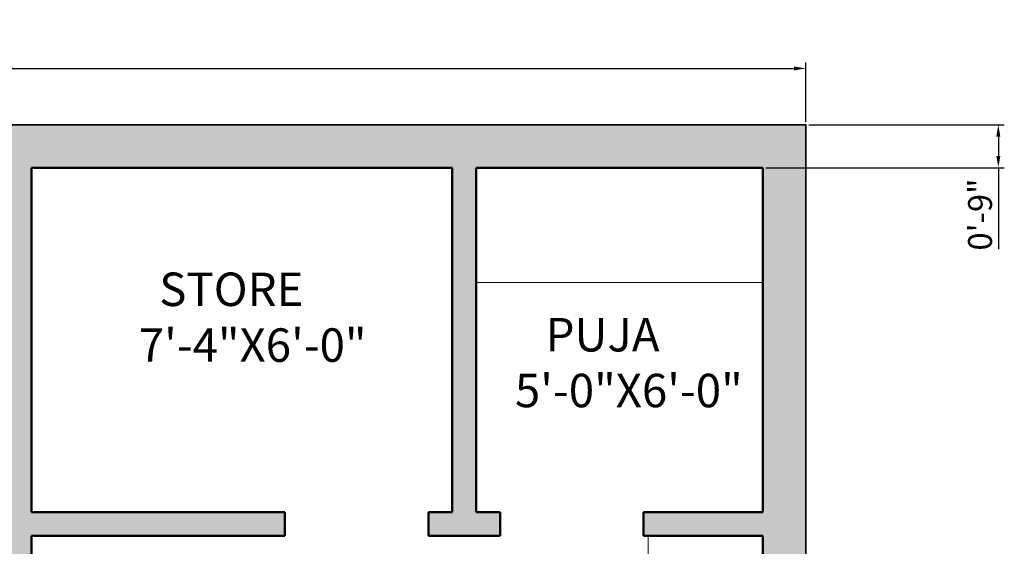
# Model space of a CAD drawing. Units: inches. Extents: x 1734 to 4011, y 1071 to 1891.
# Tile 9 of 27: x 1954 to 2160, y 1756 to 1866. Entities that reach past the tile are written whole.
import ezdxf

# ---------------------------------------------------------------- set-up
doc = ezdxf.new("R2010")
doc.units = ezdxf.units.IN
for name, color, linetype, lineweight in [('A-ANNO-DIMS', 2, 'Continuous', 18), ('A-AREA-IDEN', 3, 'Continuous', 18), ('A-FURN', 8, 'Continuous', 18), ('A-WALL', 7, 'Continuous', 50), ('A-WALL-PATT', 8, 'Continuous', 13), ('C-PROP', 1, 'Continuous', 35)]:
    doc.layers.add(name, color=color, linetype=linetype, lineweight=lineweight)
doc.styles.get("Standard").update_dxf_attribs({"font": 'arial.ttf'})
doc.dimstyles.new('ISO-25', dxfattribs={"dimtxt": 5, "dimasz": 2.5, "dimexe": 1.25, "dimexo": 0.625, "dimtad": 1, "dimdec": 1, "dimlunit": 3, "dimtxsty": 'Standard', "dimcen": 2.5, "dimclrt": 1, "dimadec": 0, "dimazin": 0, "dimtfac": 1, "dimtdec": 1, "dimtmove": 0, "dimatfit": 3, "dimfxl": 1, "dimarcsym": 0})

# ---------------------------------------------------------------- blocks, each defined once
blk = doc.blocks.new('*D14')
at = {"layer": 'A-ANNO-DIMS', "color": 0, "lineweight": -2, "transparency": 16777216}
for p, q in [((1758.65, 1844.69), (1758.65, 1857.09)), ((2118.65, 1844.69), (2118.65, 1857.09)), ((1761.15, 1855.84), (2116.15, 1855.84))]:
    blk.add_line(p, q, dxfattribs=at)
at = {"layer": 'A-ANNO-DIMS', "color": 0, "transparency": 16777216}
for points in [[(1761.15, 1856.26), (1761.15, 1855.43), (1758.65, 1855.84)], [(2116.15, 1856.26), (2116.15, 1855.43), (2118.65, 1855.84)]]:
    blk.add_solid(points, dxfattribs=at)
at = {"layer": 'Defpoints', "color": 0, "transparency": 16777216}
for p in [(2118.65, 1855.84), (1758.65, 1844.06), (2118.65, 1844.06)]:
    blk.add_point(p, dxfattribs=at)
at = {"layer": 'A-ANNO-DIMS', "color": 0, "transparency": 16777216, "insert": (1938.65, 1861.07), "char_height": 5, "attachment_point": 5}
blk.add_mtext("{\\H1.8x;30'}", dxfattribs=at)
blk = doc.blocks.new('*D104')
at = {"layer": 'A-ANNO-DIMS', "color": 0, "lineweight": -2, "transparency": 16777216}
for p, q in [((2119.27, 1844.06), (2160.15, 1844.06)), ((2158.9, 1841.56), (2158.9, 1837.56)), ((2110.27, 1835.06), (2160.15, 1835.06)), ((2158.9, 1835.06), (2158.9, 1818.02))]:
    blk.add_line(p, q, dxfattribs=at)
at = {"layer": 'A-ANNO-DIMS', "color": 0, "transparency": 16777216}
for points in [[(2158.48, 1841.56), (2159.32, 1841.56), (2158.9, 1844.06)], [(2158.48, 1837.56), (2159.32, 1837.56), (2158.9, 1835.06)]]:
    blk.add_solid(points, dxfattribs=at)
at = {"layer": 'Defpoints', "color": 0, "transparency": 16777216}
for p in [(2118.65, 1844.06), (2109.65, 1835.06), (2158.9, 1835.06)]:
    blk.add_point(p, dxfattribs=at)
at = {"layer": 'A-ANNO-DIMS', "color": 1, "transparency": 16777216, "insert": (2155.72, 1825.29), "char_height": 5, "attachment_point": 5, "rotation": 90}
blk.add_mtext('0\'-9"', dxfattribs=at)

msp = doc.modelspace()

# ---------------------------------------------------------------- hatches: boundary and pattern name
at = {"layer": 'A-WALL-PATT'}
h = msp.add_hatch(color=256, dxfattribs=at)
h.dxf.hatch_style = 1
h.paths.add_polyline_path([(1857.65, 1835.06), (1857.65, 1793.06), (1862.65, 1793.06), (1862.65, 1835.06), (1951.65, 1835.06), (1951.65, 1763.06), (1897.65, 1763.06), (1897.65, 1758.06), (1951.65, 1758.06), (1951.65, 1617.06), (1956.65, 1617.06), (1956.65, 1758.06), (2009.65, 1758.06), (2009.65, 1763.06), (1956.65, 1763.06), (1956.65, 1835.06), (2044.65, 1835.06), (2044.65, 1763.06), (2039.65, 1763.06), (2039.65, 1758.06), (2054.65, 1758.06), (2054.65, 1763.06), (2049.65, 1763.06), (2049.65, 1835.06), (2109.65, 1835.06), (2109.65, 1763.06), (2084.65, 1763.06), (2084.65, 1758.06), (2109.65, 1758.06), (2109.65, 1530.06), (2095.15, 1530.06), (2095.15, 1525.06), (2109.65, 1525.06), (2109.65, 1471.06), (2089.15, 1471.06), (2089.15, 1466.06), (2109.65, 1466.06), (2109.65, 1250.06), (2015.65, 1250.06), (2015.65, 1241.06), (2109.65, 1241.06), (2109.65, 1133.06), (1952.65, 1133.06), (1952.65, 1197.06), (1953.65, 1197.06), (1953.65, 1202.06), (1946.65, 1202.06), (1946.65, 1133.06), (1934.65, 1133.06), (1934.65, 1124.06), (2118.65, 1124.06), (2118.65, 1844.06), (1758.65, 1844.06), (1758.65, 1758.06), (1773.65, 1758.06), (1773.65, 1763.06), (1767.65, 1763.06), (1767.65, 1835.06)])
h.paths.add_polyline_path([(1803.65, 1649.06), (1812.65, 1649.06), (1812.65, 1758.06), (1867.65, 1758.06), (1867.65, 1763.06), (1797.65, 1763.06), (1797.65, 1758.06), (1803.65, 1758.06)], flags=17)
h.paths.add_polyline_path([(1803.65, 1572.06), (1956.65, 1572.06), (1956.65, 1581.06), (1951.65, 1581.06), (1951.65, 1577.06), (1812.65, 1577.06), (1812.65, 1601.06), (1803.65, 1601.06)], flags=17)
h.paths.add_polyline_path([(2044.65, 1530.06), (2044.65, 1525.06), (2059.15, 1525.06), (2059.15, 1530.06)], flags=17)
h.paths.add_polyline_path([(2009.65, 1466.06), (2035.15, 1466.06), (2035.15, 1471.06), (2014.65, 1471.06), (2014.65, 1530.06), (2009.65, 1530.06)], flags=17)
h.paths.add_polyline_path([(1896.65, 1537.06), (1896.65, 1533.06), (1901.65, 1533.06), (1901.65, 1542.06), (1803.65, 1542.06), (1803.65, 1507.06), (1812.65, 1507.06), (1812.65, 1537.06)], flags=17)
h.paths.add_polyline_path([(1906.65, 1466.06), (1906.65, 1471.06), (1901.65, 1471.06), (1901.65, 1503.06), (1896.65, 1503.06), (1896.65, 1471.06), (1812.65, 1471.06), (1812.65, 1483.06), (1803.65, 1483.06), (1803.65, 1400.06), (1812.65, 1400.06), (1812.65, 1466.06)], flags=17)
h.paths.add_polyline_path([(1951.65, 1334.06), (1909.15, 1334.06), (1909.15, 1325.06), (1956.65, 1325.06), (1956.65, 1466.06), (1961.65, 1466.06), (1961.65, 1471.06), (1942.65, 1471.06), (1942.65, 1466.06), (1951.65, 1466.06)], flags=17)
h.paths.add_polyline_path([(1812.65, 1334.06), (1812.65, 1352.06), (1803.65, 1352.06), (1803.65, 1325.06), (1855.15, 1325.06), (1855.15, 1334.06)], flags=17)
h.paths.add_polyline_path([(1956.65, 1298.06), (1956.65, 1301.06), (1947.65, 1301.06), (1947.65, 1298.06)], flags=17)
h.paths.add_polyline_path([(1967.65, 1241.06), (1967.65, 1250.06), (1947.65, 1250.06), (1947.65, 1241.06)], flags=17)

# ---------------------------------------------------------------- linework, layer by layer
at = {"layer": 'A-FURN'}
for p, q in [((2049.65, 1811.06), (2109.65, 1811.06)), ((2085.65, 1758.06), (2085.65, 1650.06)), ((2085.65, 1758.06), (2085.65, 1650.06))]:
    msp.add_line(p, q, dxfattribs=at)
at = {"layer": 'A-WALL'}
for p, q in [((1956.65, 1835.06), (2044.65, 1835.06)), ((1956.65, 1763.06), (1956.65, 1835.06)), ((2044.65, 1763.06), (2044.65, 1835.06)), ((2049.65, 1763.06), (2049.65, 1835.06)), ((2049.65, 1835.06), (2109.65, 1835.06)), ((2109.65, 1835.06), (2109.65, 1763.06)), ((1956.65, 1763.06), (2009.65, 1763.06)), ((2009.65, 1758.06), (2009.65, 1763.06)), ((2039.65, 1758.06), (2039.65, 1763.06)), ((2039.65, 1763.06), (2044.65, 1763.06)), ((2049.65, 1763.06), (2054.65, 1763.06)), ((2054.65, 1758.06), (2054.65, 1763.06)), ((2084.65, 1758.06), (2084.65, 1763.06)), ((2084.65, 1763.06), (2109.65, 1763.06)), ((1956.65, 1617.06), (1956.65, 1758.06)), ((1956.65, 1758.06), (2009.65, 1758.06)), ((2039.65, 1758.06), (2054.65, 1758.06)), ((2084.65, 1758.06), (2109.65, 1758.06)), ((2109.65, 1758.06), (2109.65, 1530.06))]:
    msp.add_line(p, q, dxfattribs=at)
at = {"layer": 'C-PROP'}
msp.add_lwpolyline([(1814.65, 1124.06), (1758.65, 1124.06), (1758.65, 1844.06), (2118.65, 1844.06), (2118.65, 1124.06), (1934.65, 1124.06)], dxfattribs=at)

# ---------------------------------------------------------------- texts
at = {"layer": 'A-AREA-IDEN', "char_height": 7, "attachment_point": 1}
for s, insert in [('  STORE\\P7\'-4"X6\'-0"', (1979.06, 1813.15)), ('   PUJA\\P5\'-0"X6\'-0"', (2057.76, 1803.65))]:
    msp.add_mtext_dynamic_manual_height_columns(s, width=86.9528, gutter_width=12.5, heights=[18.94], dxfattribs=dict(at, insert=insert))

# ---------------------------------------------------------------- dimensions: what is measured, and where the dimension line sits
at = {"layer": 'A-ANNO-DIMS'}
dim = msp.add_linear_dim(base=(2118.65, 1855.84), p1=(1758.65, 1844.06), p2=(2118.65, 1844.06), text='{\\H1.8x;<>}', dimstyle='ISO-25', override={"dimclrd": 0, "dimclre": 0, "dimclrt": 0}, dxfattribs=at)
dim.commit()
dim.dimension.update_dxf_attribs({"geometry": '*D14', "text_midpoint": (1938.65, 1861.07)})
dim = msp.add_linear_dim(base=(2158.9, 1835.06), p1=(2118.65, 1844.06), p2=(2109.65, 1835.06), angle=90, dimstyle='ISO-25', override={"dimdec": 1, "dimlfac": 1, "dimrnd": 0, "dimzin": 1, "dimdsep": 46, "dimlunit": 4, "dimfrac": 2}, dxfattribs=at)
dim.commit()
dim.dimension.update_dxf_attribs({"geometry": '*D104', "text_midpoint": (2155.72, 1825.29)})

doc.saveas('drawing.dxf')
